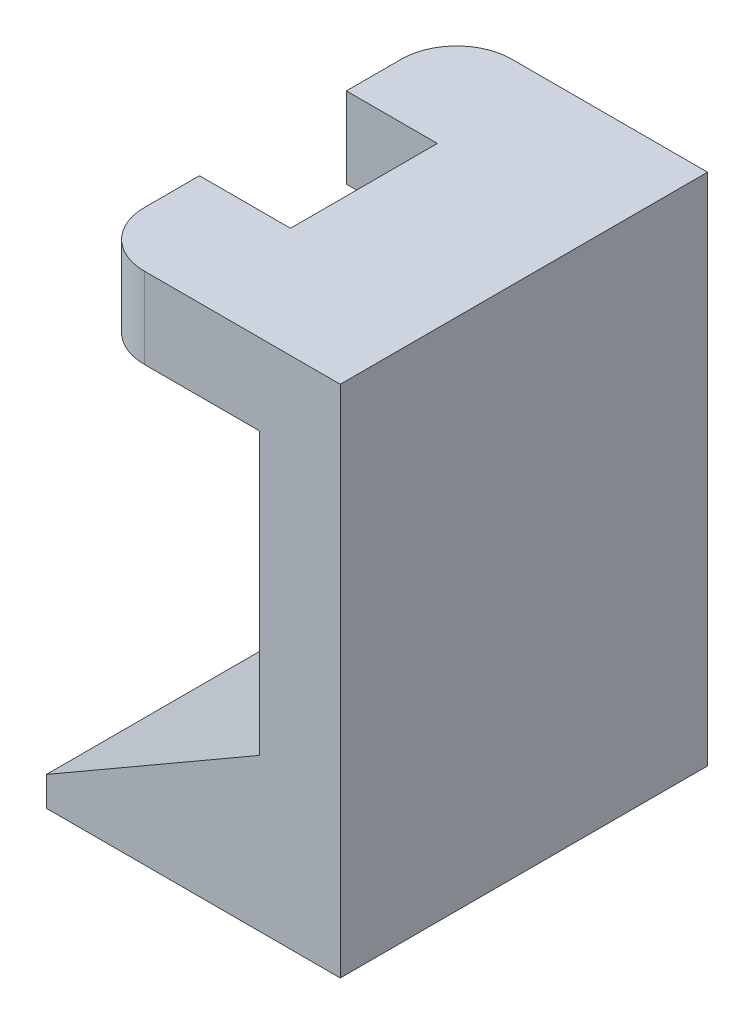
ISO-10303-21;
HEADER;
FILE_DESCRIPTION(('STEP AP214'),'2;1');
FILE_NAME('part.step','',(''),(''),'','','');
FILE_SCHEMA(('AUTOMOTIVE_DESIGN { 1 0 10303 214 1 1 1 1 }'));
ENDSEC;
DATA;
#1=APPLICATION_CONTEXT('core data for automotive mechanical design processes');
#2=APPLICATION_PROTOCOL_DEFINITION('international standard','automotive_design',2000,#1);
#3=PRODUCT_CONTEXT('',#1,'mechanical');
#4=PRODUCT('Part','Part','',(#3));
#5=PRODUCT_RELATED_PRODUCT_CATEGORY('part','',(#4));
#6=PRODUCT_DEFINITION_FORMATION('','',#4);
#7=PRODUCT_DEFINITION_CONTEXT('part definition',#1,'design');
#8=PRODUCT_DEFINITION('design','',#6,#7);
#9=PRODUCT_DEFINITION_SHAPE('','',#8);
#10=(LENGTH_UNIT() NAMED_UNIT(*) SI_UNIT(.MILLI.,.METRE.));
#11=(NAMED_UNIT(*) PLANE_ANGLE_UNIT() SI_UNIT($,.RADIAN.));
#12=(NAMED_UNIT(*) SI_UNIT($,.STERADIAN.) SOLID_ANGLE_UNIT());
#13=UNCERTAINTY_MEASURE_WITH_UNIT(LENGTH_MEASURE(1.E-05),#10,'distance_accuracy_value','');
#14=(GEOMETRIC_REPRESENTATION_CONTEXT(3) GLOBAL_UNCERTAINTY_ASSIGNED_CONTEXT((#13)) GLOBAL_UNIT_ASSIGNED_CONTEXT((#10,
#11,#12)) REPRESENTATION_CONTEXT('',''));
#15=CARTESIAN_POINT('',(0.,0.,0.));
#16=DIRECTION('',(0.,0.,1.));
#17=DIRECTION('',(1.,0.,0.));
#18=AXIS2_PLACEMENT_3D('',#15,#16,#17);
#19=CARTESIAN_POINT('',(-1.36670697030651,1.4,1.));
#20=DIRECTION('',(1.,0.,0.));
#21=DIRECTION('',(0.,0.,-1.));
#22=AXIS2_PLACEMENT_3D('',#19,#20,#21);
#23=PLANE('',#22);
#24=DIRECTION('',(0.,1.,0.));
#25=VECTOR('',#24,1.);
#26=CARTESIAN_POINT('',(-1.36670697030651,0.9,0.7));
#27=LINE('',#26,#25);
#28=CARTESIAN_POINT('',(-1.36670697030651,0.96,0.7));
#29=VERTEX_POINT('',#28);
#30=CARTESIAN_POINT('',(-1.36670697030651,1.4,0.7));
#31=VERTEX_POINT('',#30);
#32=EDGE_CURVE('E154',#29,#31,#27,.T.);
#33=ORIENTED_EDGE('',*,*,#32,.T.);
#34=DIRECTION('',(0.,0.,-1.));
#35=VECTOR('',#34,1.);
#36=CARTESIAN_POINT('',(-1.36670697030651,1.4,1.));
#37=LINE('',#36,#35);
#38=CARTESIAN_POINT('',(-1.36670697030651,1.4,0.399987472869384));
#39=VERTEX_POINT('',#38);
#40=EDGE_CURVE('E159',#31,#39,#37,.T.);
#41=ORIENTED_EDGE('',*,*,#40,.T.);
#42=DIRECTION('',(0.,1.,0.));
#43=VECTOR('',#42,1.);
#44=CARTESIAN_POINT('',(-1.36670697030651,0.9,0.399987472869384));
#45=LINE('',#44,#43);
#46=CARTESIAN_POINT('',(-1.36670697030651,0.96,0.399987472869384));
#47=VERTEX_POINT('',#46);
#48=EDGE_CURVE('E255',#47,#39,#45,.T.);
#49=ORIENTED_EDGE('',*,*,#48,.F.);
#50=DIRECTION('',(0.,0.,-1.));
#51=VECTOR('',#50,1.);
#52=CARTESIAN_POINT('',(-1.36670697030651,0.96,1.));
#53=LINE('',#52,#51);
#54=EDGE_CURVE('E161',#29,#47,#53,.T.);
#55=ORIENTED_EDGE('',*,*,#54,.F.);
#56=EDGE_LOOP('',(#33,#41,#49,#55));
#57=FACE_BOUND('',#56,.T.);
#58=ADVANCED_FACE('F39',(#57),#23,.F.);
#59=CARTESIAN_POINT('',(-1.36670697030651,1.4,-0.4));
#60=VERTEX_POINT('',#59);
#61=CARTESIAN_POINT('',(-1.36670697030651,1.4,-0.7));
#62=VERTEX_POINT('',#61);
#63=EDGE_CURVE('E151',#60,#62,#37,.T.);
#64=ORIENTED_EDGE('',*,*,#63,.T.);
#65=DIRECTION('',(0.,1.,0.));
#66=VECTOR('',#65,1.);
#67=CARTESIAN_POINT('',(-1.36670697030651,0.9,-0.7));
#68=LINE('',#67,#66);
#69=CARTESIAN_POINT('',(-1.36670697030651,0.96,-0.7));
#70=VERTEX_POINT('',#69);
#71=EDGE_CURVE('E139',#70,#62,#68,.T.);
#72=ORIENTED_EDGE('',*,*,#71,.F.);
#73=CARTESIAN_POINT('',(-1.36670697030651,0.96,-0.4));
#74=VERTEX_POINT('',#73);
#75=EDGE_CURVE('E163',#74,#70,#53,.T.);
#76=ORIENTED_EDGE('',*,*,#75,.F.);
#77=DIRECTION('',(0.,1.,0.));
#78=VECTOR('',#77,1.);
#79=CARTESIAN_POINT('',(-1.36670697030651,0.9,-0.4));
#80=LINE('',#79,#78);
#81=EDGE_CURVE('E157',#74,#60,#80,.T.);
#82=ORIENTED_EDGE('',*,*,#81,.T.);
#83=EDGE_LOOP('',(#64,#72,#76,#82));
#84=FACE_BOUND('',#83,.T.);
#85=ADVANCED_FACE('F158',(#84),#23,.F.);
#86=CARTESIAN_POINT('',(0.,0.,1.));
#87=DIRECTION('',(-1.,0.,0.));
#88=DIRECTION('',(0.,0.,1.));
#89=AXIS2_PLACEMENT_3D('',#86,#87,#88);
#90=PLANE('',#89);
#91=DIRECTION('',(0.,1.,0.));
#92=VECTOR('',#91,1.);
#93=CARTESIAN_POINT('',(0.,0.,-1.));
#94=LINE('',#93,#92);
#95=CARTESIAN_POINT('',(0.,-1.4,-1.));
#96=VERTEX_POINT('',#95);
#97=CARTESIAN_POINT('',(0.,1.4,-1.));
#98=VERTEX_POINT('',#97);
#99=EDGE_CURVE('E171',#96,#98,#94,.T.);
#100=ORIENTED_EDGE('',*,*,#99,.T.);
#101=DIRECTION('',(0.,0.,-1.));
#102=VECTOR('',#101,1.);
#103=CARTESIAN_POINT('',(0.,1.4,1.));
#104=LINE('',#103,#102);
#105=CARTESIAN_POINT('',(0.,1.4,1.));
#106=VERTEX_POINT('',#105);
#107=EDGE_CURVE('E162',#106,#98,#104,.T.);
#108=ORIENTED_EDGE('',*,*,#107,.F.);
#109=DIRECTION('',(0.,1.,0.));
#110=VECTOR('',#109,1.);
#111=CARTESIAN_POINT('',(0.,0.,1.));
#112=LINE('',#111,#110);
#113=CARTESIAN_POINT('',(0.,-1.4,1.));
#114=VERTEX_POINT('',#113);
#115=EDGE_CURVE('E206',#114,#106,#112,.T.);
#116=ORIENTED_EDGE('',*,*,#115,.F.);
#117=DIRECTION('',(0.,0.,-1.));
#118=VECTOR('',#117,1.);
#119=CARTESIAN_POINT('',(0.,-1.4,1.));
#120=LINE('',#119,#118);
#121=EDGE_CURVE('E210',#114,#96,#120,.T.);
#122=ORIENTED_EDGE('',*,*,#121,.T.);
#123=EDGE_LOOP('',(#100,#108,#116,#122));
#124=FACE_BOUND('',#123,.T.);
#125=ADVANCED_FACE('F41',(#124),#90,.F.);
#126=CARTESIAN_POINT('',(0.,1.4,1.));
#127=DIRECTION('',(0.,-1.,0.));
#128=DIRECTION('',(1.,0.,0.));
#129=AXIS2_PLACEMENT_3D('',#126,#127,#128);
#130=PLANE('',#129);
#131=DIRECTION('',(-1.,0.,0.));
#132=VECTOR('',#131,1.);
#133=CARTESIAN_POINT('',(0.,1.4,-1.));
#134=LINE('',#133,#132);
#135=CARTESIAN_POINT('',(-1.06670697030651,1.4,-1.));
#136=VERTEX_POINT('',#135);
#137=EDGE_CURVE('E152',#98,#136,#134,.T.);
#138=ORIENTED_EDGE('',*,*,#137,.T.);
#139=CARTESIAN_POINT('',(-1.06670697030651,1.4,-0.7));
#140=DIRECTION('',(0.,-1.,0.));
#141=DIRECTION('',(-1.,0.,0.));
#142=AXIS2_PLACEMENT_3D('',#139,#140,#141);
#143=CIRCLE('',#142,0.3);
#144=EDGE_CURVE('E63',#62,#136,#143,.T.);
#145=ORIENTED_EDGE('',*,*,#144,.F.);
#146=ORIENTED_EDGE('',*,*,#63,.F.);
#147=DIRECTION('',(-1.,0.,0.));
#148=VECTOR('',#147,1.);
#149=CARTESIAN_POINT('',(0.,1.4,-0.4));
#150=LINE('',#149,#148);
#151=CARTESIAN_POINT('',(-0.871183939376764,1.4,-0.4));
#152=VERTEX_POINT('',#151);
#153=EDGE_CURVE('E256',#152,#60,#150,.T.);
#154=ORIENTED_EDGE('',*,*,#153,.F.);
#155=DIRECTION('',(0.,0.,1.));
#156=VECTOR('',#155,1.);
#157=CARTESIAN_POINT('',(-0.871183939376764,1.4,0.));
#158=LINE('',#157,#156);
#159=CARTESIAN_POINT('',(-0.871183939376764,1.4,0.399987472869384));
#160=VERTEX_POINT('',#159);
#161=EDGE_CURVE('E262',#152,#160,#158,.T.);
#162=ORIENTED_EDGE('',*,*,#161,.T.);
#163=DIRECTION('',(1.,0.,0.));
#164=VECTOR('',#163,1.);
#165=CARTESIAN_POINT('',(0.,1.4,0.399987472869385));
#166=LINE('',#165,#164);
#167=EDGE_CURVE('E270',#39,#160,#166,.T.);
#168=ORIENTED_EDGE('',*,*,#167,.F.);
#169=ORIENTED_EDGE('',*,*,#40,.F.);
#170=CARTESIAN_POINT('',(-1.06670697030651,1.4,0.7));
#171=DIRECTION('',(0.,-1.,0.));
#172=DIRECTION('',(1.,0.,0.));
#173=AXIS2_PLACEMENT_3D('',#170,#171,#172);
#174=CIRCLE('',#173,0.3);
#175=CARTESIAN_POINT('',(-1.06670697030651,1.4,1.));
#176=VERTEX_POINT('',#175);
#177=EDGE_CURVE('E247',#176,#31,#174,.T.);
#178=ORIENTED_EDGE('',*,*,#177,.F.);
#179=DIRECTION('',(-1.,0.,0.));
#180=VECTOR('',#179,1.);
#181=CARTESIAN_POINT('',(0.,1.4,1.));
#182=LINE('',#181,#180);
#183=EDGE_CURVE('E229',#106,#176,#182,.T.);
#184=ORIENTED_EDGE('',*,*,#183,.F.);
#185=ORIENTED_EDGE('',*,*,#107,.T.);
#186=EDGE_LOOP('',(#138,#145,#146,#154,#162,#168,#169,#178,#184,#185));
#187=FACE_BOUND('',#186,.T.);
#188=ADVANCED_FACE('F149',(#187),#130,.F.);
#189=CARTESIAN_POINT('',(-1.36670697030651,0.96,1.));
#190=DIRECTION('',(0.,1.,0.));
#191=DIRECTION('',(0.,0.,1.));
#192=AXIS2_PLACEMENT_3D('',#189,#190,#191);
#193=PLANE('',#192);
#194=ORIENTED_EDGE('',*,*,#75,.T.);
#195=CARTESIAN_POINT('',(-1.06670697030651,0.96,-0.7));
#196=DIRECTION('',(0.,1.,0.));
#197=DIRECTION('',(0.,0.,1.));
#198=AXIS2_PLACEMENT_3D('',#195,#196,#197);
#199=CIRCLE('',#198,0.3);
#200=CARTESIAN_POINT('',(-1.06670697030651,0.96,-1.));
#201=VERTEX_POINT('',#200);
#202=EDGE_CURVE('E136',#70,#201,#199,.F.);
#203=ORIENTED_EDGE('',*,*,#202,.T.);
#204=DIRECTION('',(1.,0.,0.));
#205=VECTOR('',#204,1.);
#206=CARTESIAN_POINT('',(-1.36670697030651,0.96,-1.));
#207=LINE('',#206,#205);
#208=CARTESIAN_POINT('',(-0.44,0.96,-1.));
#209=VERTEX_POINT('',#208);
#210=EDGE_CURVE('E190',#201,#209,#207,.T.);
#211=ORIENTED_EDGE('',*,*,#210,.T.);
#212=DIRECTION('',(0.,0.,-1.));
#213=VECTOR('',#212,1.);
#214=CARTESIAN_POINT('',(-0.44,0.96,1.));
#215=LINE('',#214,#213);
#216=CARTESIAN_POINT('',(-0.44,0.96,1.));
#217=VERTEX_POINT('',#216);
#218=EDGE_CURVE('E218',#217,#209,#215,.T.);
#219=ORIENTED_EDGE('',*,*,#218,.F.);
#220=DIRECTION('',(1.,0.,0.));
#221=VECTOR('',#220,1.);
#222=CARTESIAN_POINT('',(-1.36670697030651,0.96,1.));
#223=LINE('',#222,#221);
#224=CARTESIAN_POINT('',(-1.06670697030651,0.96,1.));
#225=VERTEX_POINT('',#224);
#226=EDGE_CURVE('E228',#225,#217,#223,.T.);
#227=ORIENTED_EDGE('',*,*,#226,.F.);
#228=CARTESIAN_POINT('',(-1.06670697030651,0.96,0.7));
#229=DIRECTION('',(0.,1.,0.));
#230=DIRECTION('',(0.,0.,1.));
#231=AXIS2_PLACEMENT_3D('',#228,#229,#230);
#232=CIRCLE('',#231,0.3);
#233=EDGE_CURVE('E53',#225,#29,#232,.F.);
#234=ORIENTED_EDGE('',*,*,#233,.T.);
#235=ORIENTED_EDGE('',*,*,#54,.T.);
#236=DIRECTION('',(1.,0.,0.));
#237=VECTOR('',#236,1.);
#238=CARTESIAN_POINT('',(-1.36670697030651,0.96,0.399987472869384));
#239=LINE('',#238,#237);
#240=CARTESIAN_POINT('',(-0.871183939376764,0.96,0.399987472869384));
#241=VERTEX_POINT('',#240);
#242=EDGE_CURVE('E166',#47,#241,#239,.T.);
#243=ORIENTED_EDGE('',*,*,#242,.T.);
#244=DIRECTION('',(0.,0.,1.));
#245=VECTOR('',#244,1.);
#246=CARTESIAN_POINT('',(-0.871183939376764,0.96,1.));
#247=LINE('',#246,#245);
#248=CARTESIAN_POINT('',(-0.871183939376764,0.96,-0.4));
#249=VERTEX_POINT('',#248);
#250=EDGE_CURVE('E179',#249,#241,#247,.T.);
#251=ORIENTED_EDGE('',*,*,#250,.F.);
#252=DIRECTION('',(-1.,0.,0.));
#253=VECTOR('',#252,1.);
#254=CARTESIAN_POINT('',(-1.36670697030651,0.96,-0.4));
#255=LINE('',#254,#253);
#256=EDGE_CURVE('E176',#249,#74,#255,.T.);
#257=ORIENTED_EDGE('',*,*,#256,.T.);
#258=EDGE_LOOP('',(#194,#203,#211,#219,#227,#234,#235,#243,#251,#257));
#259=FACE_BOUND('',#258,.T.);
#260=ADVANCED_FACE('F183',(#259),#193,.F.);
#261=CARTESIAN_POINT('',(-0.44,0.96,1.));
#262=DIRECTION('',(1.,0.,0.));
#263=DIRECTION('',(0.,1.,0.));
#264=AXIS2_PLACEMENT_3D('',#261,#262,#263);
#265=PLANE('',#264);
#266=DIRECTION('',(0.,-1.,0.));
#267=VECTOR('',#266,1.);
#268=CARTESIAN_POINT('',(-0.44,0.96,-1.));
#269=LINE('',#268,#267);
#270=CARTESIAN_POINT('',(-0.44,-0.570273687740032,-1.));
#271=VERTEX_POINT('',#270);
#272=EDGE_CURVE('E192',#209,#271,#269,.T.);
#273=ORIENTED_EDGE('',*,*,#272,.T.);
#274=DIRECTION('',(0.,0.,-1.));
#275=VECTOR('',#274,1.);
#276=CARTESIAN_POINT('',(-0.44,-0.570273687740032,1.));
#277=LINE('',#276,#275);
#278=CARTESIAN_POINT('',(-0.44,-0.570273687740032,1.));
#279=VERTEX_POINT('',#278);
#280=EDGE_CURVE('E220',#279,#271,#277,.T.);
#281=ORIENTED_EDGE('',*,*,#280,.F.);
#282=DIRECTION('',(0.,-1.,0.));
#283=VECTOR('',#282,1.);
#284=CARTESIAN_POINT('',(-0.44,0.96,1.));
#285=LINE('',#284,#283);
#286=EDGE_CURVE('E221',#217,#279,#285,.T.);
#287=ORIENTED_EDGE('',*,*,#286,.F.);
#288=ORIENTED_EDGE('',*,*,#218,.T.);
#289=EDGE_LOOP('',(#273,#281,#287,#288));
#290=FACE_BOUND('',#289,.T.);
#291=ADVANCED_FACE('F225',(#290),#265,.F.);
#292=CARTESIAN_POINT('',(-1.6,-1.24,1.));
#293=DIRECTION('',(0.500000000000001,-0.866025403784438,0.));
#294=DIRECTION('',(0.866025403784438,0.500000000000001,0.));
#295=AXIS2_PLACEMENT_3D('',#292,#293,#294);
#296=PLANE('',#295);
#297=CARTESIAN_POINT('',(-0.99355464638751,-0.88986861184303,0.));
#298=DIRECTION('',(-0.500000000000001,0.866025403784438,0.));
#299=DIRECTION('',(-0.866025403784438,-0.500000000000001,0.));
#300=AXIS2_PLACEMENT_3D('',#297,#298,#299);
#301=CIRCLE('',#300,0.2);
#302=CARTESIAN_POINT('',(-1.1667597271444,-0.989868611843031,0.));
#303=VERTEX_POINT('',#302);
#304=EDGE_CURVE('E174',#303,#303,#301,.T.);
#305=ORIENTED_EDGE('',*,*,#304,.F.);
#306=EDGE_LOOP('',(#305));
#307=FACE_BOUND('',#306,.T.);
#308=DIRECTION('',(-0.866025403784438,-0.500000000000001,0.));
#309=VECTOR('',#308,1.);
#310=CARTESIAN_POINT('',(-1.6,-1.24,-1.));
#311=LINE('',#310,#309);
#312=CARTESIAN_POINT('',(-1.6,-1.24,-1.));
#313=VERTEX_POINT('',#312);
#314=EDGE_CURVE('E191',#271,#313,#311,.T.);
#315=ORIENTED_EDGE('',*,*,#314,.T.);
#316=DIRECTION('',(0.,0.,-1.));
#317=VECTOR('',#316,1.);
#318=CARTESIAN_POINT('',(-1.6,-1.24,1.));
#319=LINE('',#318,#317);
#320=CARTESIAN_POINT('',(-1.6,-1.24,1.));
#321=VERTEX_POINT('',#320);
#322=EDGE_CURVE('E212',#321,#313,#319,.T.);
#323=ORIENTED_EDGE('',*,*,#322,.F.);
#324=DIRECTION('',(-0.866025403784438,-0.500000000000001,0.));
#325=VECTOR('',#324,1.);
#326=CARTESIAN_POINT('',(-1.6,-1.24,1.));
#327=LINE('',#326,#325);
#328=EDGE_CURVE('E233',#279,#321,#327,.T.);
#329=ORIENTED_EDGE('',*,*,#328,.F.);
#330=ORIENTED_EDGE('',*,*,#280,.T.);
#331=EDGE_LOOP('',(#315,#323,#329,#330));
#332=FACE_BOUND('',#331,.T.);
#333=ADVANCED_FACE('F319',(#307,#332),#296,.F.);
#334=CARTESIAN_POINT('',(-1.6,-1.4,1.));
#335=DIRECTION('',(1.,0.,0.));
#336=DIRECTION('',(0.,0.,-1.));
#337=AXIS2_PLACEMENT_3D('',#334,#335,#336);
#338=PLANE('',#337);
#339=DIRECTION('',(0.,-1.,0.));
#340=VECTOR('',#339,1.);
#341=CARTESIAN_POINT('',(-1.6,-1.4,-1.));
#342=LINE('',#341,#340);
#343=CARTESIAN_POINT('',(-1.6,-1.4,-1.));
#344=VERTEX_POINT('',#343);
#345=EDGE_CURVE('E203',#313,#344,#342,.T.);
#346=ORIENTED_EDGE('',*,*,#345,.T.);
#347=DIRECTION('',(0.,0.,-1.));
#348=VECTOR('',#347,1.);
#349=CARTESIAN_POINT('',(-1.6,-1.4,1.));
#350=LINE('',#349,#348);
#351=CARTESIAN_POINT('',(-1.6,-1.4,1.));
#352=VERTEX_POINT('',#351);
#353=EDGE_CURVE('E209',#352,#344,#350,.T.);
#354=ORIENTED_EDGE('',*,*,#353,.F.);
#355=DIRECTION('',(0.,-1.,0.));
#356=VECTOR('',#355,1.);
#357=CARTESIAN_POINT('',(-1.6,-1.4,1.));
#358=LINE('',#357,#356);
#359=EDGE_CURVE('E236',#321,#352,#358,.T.);
#360=ORIENTED_EDGE('',*,*,#359,.F.);
#361=ORIENTED_EDGE('',*,*,#322,.T.);
#362=EDGE_LOOP('',(#346,#354,#360,#361));
#363=FACE_BOUND('',#362,.T.);
#364=ADVANCED_FACE('F326',(#363),#338,.F.);
#365=CARTESIAN_POINT('',(0.,-1.4,1.));
#366=DIRECTION('',(0.,1.,0.));
#367=DIRECTION('',(0.,0.,1.));
#368=AXIS2_PLACEMENT_3D('',#365,#366,#367);
#369=PLANE('',#368);
#370=CARTESIAN_POINT('',(-0.699030152113005,-1.4,0.));
#371=DIRECTION('',(0.,1.,0.));
#372=DIRECTION('',(-1.,0.,0.));
#373=AXIS2_PLACEMENT_3D('',#370,#371,#372);
#374=ELLIPSE('',#373,0.230940107675851,0.2);
#375=CARTESIAN_POINT('',(-0.929970259788856,-1.4,0.));
#376=VERTEX_POINT('',#375);
#377=EDGE_CURVE('E168',#376,#376,#374,.T.);
#378=ORIENTED_EDGE('',*,*,#377,.T.);
#379=EDGE_LOOP('',(#378));
#380=FACE_BOUND('',#379,.T.);
#381=DIRECTION('',(1.,0.,0.));
#382=VECTOR('',#381,1.);
#383=CARTESIAN_POINT('',(0.,-1.4,-1.));
#384=LINE('',#383,#382);
#385=EDGE_CURVE('E201',#344,#96,#384,.T.);
#386=ORIENTED_EDGE('',*,*,#385,.T.);
#387=ORIENTED_EDGE('',*,*,#121,.F.);
#388=DIRECTION('',(1.,0.,0.));
#389=VECTOR('',#388,1.);
#390=CARTESIAN_POINT('',(0.,-1.4,1.));
#391=LINE('',#390,#389);
#392=EDGE_CURVE('E211',#352,#114,#391,.T.);
#393=ORIENTED_EDGE('',*,*,#392,.F.);
#394=ORIENTED_EDGE('',*,*,#353,.T.);
#395=EDGE_LOOP('',(#386,#387,#393,#394));
#396=FACE_BOUND('',#395,.T.);
#397=ADVANCED_FACE('F329',(#380,#396),#369,.F.);
#398=CARTESIAN_POINT('',(0.,0.,1.));
#399=DIRECTION('',(0.,0.,-1.));
#400=DIRECTION('',(-1.,0.,0.));
#401=AXIS2_PLACEMENT_3D('',#398,#399,#400);
#402=PLANE('',#401);
#403=ORIENTED_EDGE('',*,*,#183,.T.);
#404=DIRECTION('',(0.,1.,0.));
#405=VECTOR('',#404,1.);
#406=CARTESIAN_POINT('',(-1.06670697030651,0.9,1.));
#407=LINE('',#406,#405);
#408=EDGE_CURVE('E11',#176,#225,#407,.F.);
#409=ORIENTED_EDGE('',*,*,#408,.T.);
#410=ORIENTED_EDGE('',*,*,#226,.T.);
#411=ORIENTED_EDGE('',*,*,#286,.T.);
#412=ORIENTED_EDGE('',*,*,#328,.T.);
#413=ORIENTED_EDGE('',*,*,#359,.T.);
#414=ORIENTED_EDGE('',*,*,#392,.T.);
#415=ORIENTED_EDGE('',*,*,#115,.T.);
#416=EDGE_LOOP('',(#403,#409,#410,#411,#412,#413,#414,#415));
#417=FACE_BOUND('',#416,.T.);
#418=ADVANCED_FACE('F250',(#417),#402,.F.);
#419=CARTESIAN_POINT('',(0.,0.,-1.));
#420=DIRECTION('',(0.,0.,-1.));
#421=DIRECTION('',(-1.,0.,0.));
#422=AXIS2_PLACEMENT_3D('',#419,#420,#421);
#423=PLANE('',#422);
#424=DIRECTION('',(0.,1.,0.));
#425=VECTOR('',#424,1.);
#426=CARTESIAN_POINT('',(-1.06670697030651,0.9,-1.));
#427=LINE('',#426,#425);
#428=EDGE_CURVE('E50',#136,#201,#427,.F.);
#429=ORIENTED_EDGE('',*,*,#428,.F.);
#430=ORIENTED_EDGE('',*,*,#137,.F.);
#431=ORIENTED_EDGE('',*,*,#99,.F.);
#432=ORIENTED_EDGE('',*,*,#385,.F.);
#433=ORIENTED_EDGE('',*,*,#345,.F.);
#434=ORIENTED_EDGE('',*,*,#314,.F.);
#435=ORIENTED_EDGE('',*,*,#272,.F.);
#436=ORIENTED_EDGE('',*,*,#210,.F.);
#437=EDGE_LOOP('',(#429,#430,#431,#432,#433,#434,#435,#436));
#438=FACE_BOUND('',#437,.T.);
#439=ADVANCED_FACE('F193',(#438),#423,.T.);
#440=CARTESIAN_POINT('',(0.00644535361249226,-2.62191941941191,0.));
#441=DIRECTION('',(-0.500000000000001,0.866025403784438,0.));
#442=DIRECTION('',(-0.866025403784438,-0.500000000000001,0.));
#443=AXIS2_PLACEMENT_3D('',#440,#441,#442);
#444=CYLINDRICAL_SURFACE('',#443,0.2);
#445=ORIENTED_EDGE('',*,*,#304,.T.);
#446=EDGE_LOOP('',(#445));
#447=FACE_BOUND('',#446,.T.);
#448=ORIENTED_EDGE('',*,*,#377,.F.);
#449=EDGE_LOOP('',(#448));
#450=FACE_BOUND('',#449,.T.);
#451=ADVANCED_FACE('F287',(#447,#450),#444,.F.);
#452=CARTESIAN_POINT('',(0.,0.9,-0.4));
#453=DIRECTION('',(0.,0.,-1.));
#454=DIRECTION('',(-1.,0.,0.));
#455=AXIS2_PLACEMENT_3D('',#452,#453,#454);
#456=PLANE('',#455);
#457=DIRECTION('',(0.,1.,0.));
#458=VECTOR('',#457,1.);
#459=CARTESIAN_POINT('',(-0.871183939376764,0.9,-0.4));
#460=LINE('',#459,#458);
#461=EDGE_CURVE('E257',#249,#152,#460,.T.);
#462=ORIENTED_EDGE('',*,*,#461,.T.);
#463=ORIENTED_EDGE('',*,*,#153,.T.);
#464=ORIENTED_EDGE('',*,*,#81,.F.);
#465=ORIENTED_EDGE('',*,*,#256,.F.);
#466=EDGE_LOOP('',(#462,#463,#464,#465));
#467=FACE_BOUND('',#466,.T.);
#468=ADVANCED_FACE('F288',(#467),#456,.F.);
#469=CARTESIAN_POINT('',(-0.871183939376764,0.9,0.));
#470=DIRECTION('',(-1.,0.,0.));
#471=DIRECTION('',(0.,-1.,0.));
#472=AXIS2_PLACEMENT_3D('',#469,#470,#471);
#473=PLANE('',#472);
#474=ORIENTED_EDGE('',*,*,#250,.T.);
#475=DIRECTION('',(0.,1.,0.));
#476=VECTOR('',#475,1.);
#477=CARTESIAN_POINT('',(-0.871183939376764,0.9,0.399987472869384));
#478=LINE('',#477,#476);
#479=EDGE_CURVE('E260',#241,#160,#478,.T.);
#480=ORIENTED_EDGE('',*,*,#479,.T.);
#481=ORIENTED_EDGE('',*,*,#161,.F.);
#482=ORIENTED_EDGE('',*,*,#461,.F.);
#483=EDGE_LOOP('',(#474,#480,#481,#482));
#484=FACE_BOUND('',#483,.T.);
#485=ADVANCED_FACE('F284',(#484),#473,.T.);
#486=CARTESIAN_POINT('',(0.,0.9,0.399987472869385));
#487=DIRECTION('',(0.,0.,1.));
#488=DIRECTION('',(1.,0.,0.));
#489=AXIS2_PLACEMENT_3D('',#486,#487,#488);
#490=PLANE('',#489);
#491=ORIENTED_EDGE('',*,*,#48,.T.);
#492=ORIENTED_EDGE('',*,*,#167,.T.);
#493=ORIENTED_EDGE('',*,*,#479,.F.);
#494=ORIENTED_EDGE('',*,*,#242,.F.);
#495=EDGE_LOOP('',(#491,#492,#493,#494));
#496=FACE_BOUND('',#495,.T.);
#497=ADVANCED_FACE('F276',(#496),#490,.F.);
#498=CARTESIAN_POINT('',(-1.06670697030651,0.9,-0.7));
#499=DIRECTION('',(0.,1.,0.));
#500=DIRECTION('',(-1.,0.,0.));
#501=AXIS2_PLACEMENT_3D('',#498,#499,#500);
#502=CYLINDRICAL_SURFACE('',#501,0.3);
#503=ORIENTED_EDGE('',*,*,#71,.T.);
#504=ORIENTED_EDGE('',*,*,#144,.T.);
#505=ORIENTED_EDGE('',*,*,#428,.T.);
#506=ORIENTED_EDGE('',*,*,#202,.F.);
#507=EDGE_LOOP('',(#503,#504,#505,#506));
#508=FACE_BOUND('',#507,.T.);
#509=ADVANCED_FACE('F137',(#508),#502,.T.);
#510=CARTESIAN_POINT('',(-1.06670697030651,0.9,0.7));
#511=DIRECTION('',(0.,1.,0.));
#512=DIRECTION('',(-1.,0.,0.));
#513=AXIS2_PLACEMENT_3D('',#510,#511,#512);
#514=CYLINDRICAL_SURFACE('',#513,0.3);
#515=ORIENTED_EDGE('',*,*,#408,.F.);
#516=ORIENTED_EDGE('',*,*,#177,.T.);
#517=ORIENTED_EDGE('',*,*,#32,.F.);
#518=ORIENTED_EDGE('',*,*,#233,.F.);
#519=EDGE_LOOP('',(#515,#516,#517,#518));
#520=FACE_BOUND('',#519,.T.);
#521=ADVANCED_FACE('F272',(#520),#514,.T.);
#522=CLOSED_SHELL('',(#58,#85,#125,#188,#260,#291,#333,#364,#397,#418,#439,#451,#468,#485,#497,
#509,#521));
#523=MANIFOLD_SOLID_BREP('B2',#522);
#524=ADVANCED_BREP_SHAPE_REPRESENTATION('',(#18,#523),#14);
#525=SHAPE_DEFINITION_REPRESENTATION(#9,#524);
ENDSEC;
END-ISO-10303-21;
